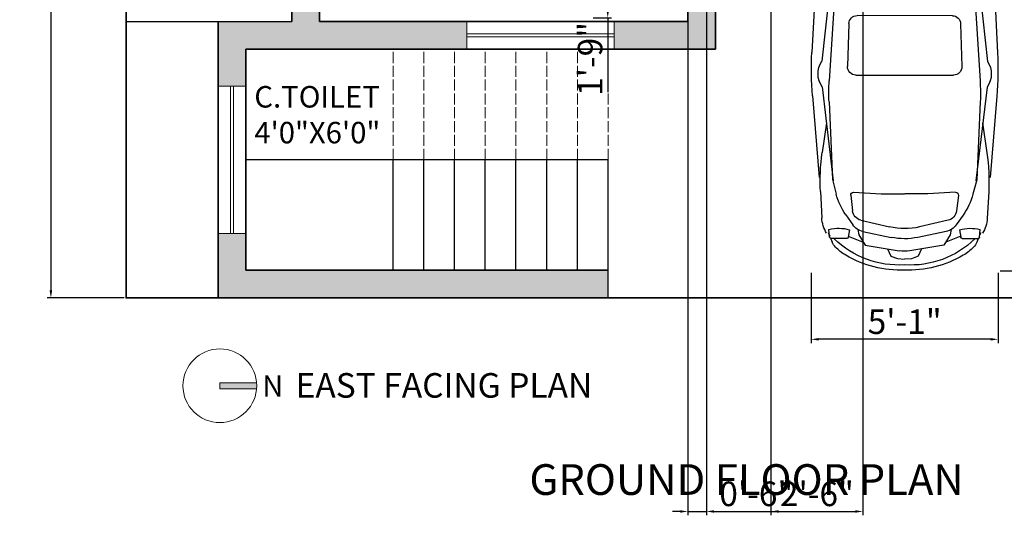
# Model space of a CAD drawing. Units: inches. Extents: x 4732 to 5926, y 2665 to 3255.
# Tile 1 of 8: x 4784 to 5104, y 2665 to 2827. Entities that reach past the tile are written whole.
import ezdxf

# ---------------------------------------------------------------- set-up
doc = ezdxf.new("R2010")
doc.units = ezdxf.units.IN
doc.linetypes.add('ACAD_ISO02W100', pattern=[15, 12, -3])
for name, color, linetype, lineweight in [('A-ANNO-DIMS', 2, 'Continuous', 18), ('A-ANNO-SYMB', 7, 'Continuous', 18), ('A-ANNO-TITL', 7, 'Continuous', 25), ('A-AREA-IDEN', 7, 'Continuous', 18), ('A-FLOR', 7, 'Continuous', 25), ('A-FLOR-STRS', 7, 'Continuous', 25), ('A-FLOR-STRS-HIDN', 8, 'ACAD_ISO02W100', 18), ('A-GLAZ', 4, 'Continuous', 18), ('A-SITE-VEHS', 8, 'Continuous', 13), ('A-WALL', 7, 'Continuous', 35), ('A-WALL-PATT', 8, 'Continuous', 13), ('C-PROP', 7, 'Continuous', 35)]:
    doc.layers.add(name, color=color, linetype=linetype, lineweight=lineweight)
doc.layers.add('L9012X$0', color=2, linetype='Continuous')
doc.styles.get("Standard").update_dxf_attribs({"font": 'arial.ttf'})
doc.dimstyles.new('ISO-25', dxfattribs={"dimtxt": 8, "dimasz": 2.5, "dimexe": 1.25, "dimexo": 0.625, "dimtad": 1, "dimdec": 1, "dimlunit": 3, "dimtxsty": 'Standard', "dimcen": 2.5, "dimadec": 0, "dimazin": 0, "dimtfac": 1, "dimtdec": 1, "dimtmove": 0, "dimatfit": 3, "dimfxl": 1, "dimarcsym": 0})

# ---------------------------------------------------------------- blocks, each defined once
blk = doc.blocks.new('A1099DC')
at = {"color": 0, "linetype": 'ByBlock'}
for p, q in [((1279.298465, 804.448389), (2201.430588, 851.890505)), ((2602.736326, 846.078152), (3356.693814, 785.353187)), ((272.228253, 749.073842), (265.114727, 718.465169)), ((1475.52921, 670.226262), (2282.402739, 758.004075)), ((2519.280414, 756.817792), (3387.476361, 653.818028)), ((2851.341839, 715.213377), (3126.60716, 755.701993)), ((3488.458929, 772.663345), (3732.658862, 759.86454)), ((139.051458, 595.027331), (190.951238, 683.213377)), ((179.200345, 564.515703), (190.951238, 709.631982)), ((398.733388, 644.315148), (411.280494, 678.748261)), ((411.280494, 678.748261), (588.616917, 641.417897)), ((1482.852352, 674.283145), (1175.286956, 622.180789)), ((1494.603245, 682.841284), (1678.210958, 641.166865)), ((1678.210958, 641.166865), (2462.684993, 690.847736)), ((2656.476214, 692.831247), (3376.704709, 662.004075)), ((3376.704709, 662.004075), (3510.708679, 626.736433)), ((3909.27561, 688.812956), (3837.725727, 693.401722)), ((3867.794139, 700.329656), (3900.059395, 686.767505)), ((3921.162781, 527.618662), (3921.162781, 676.138994)), ((3925.383812, 676.122818), (3955.306409, 663.545364)), ((92.537504, 388.14361), (139.051458, 595.027331)), ((236.043912, 551.980927), (179.200345, 564.515703)), ((405.405047, 577.538958), (396.874865, 615.894428)), ((589.014326, 626.599587), (405.405047, 577.538958)), ((1300.814287, 466.658131), (1445.712032, 613.104998)), ((1465.665584, 620.56924), (1602.893878, 610.287296)), ((1626.354615, 583.507504), (1602.652901, 169.222264)), ((229.117398, 477.634662), (225.714299, 427.957563)), ((1933.148906, 509.557888), (2330.980062, 522.200075)), ((3493.960271, 465.734554), (3507.923021, 209.166865)), ((3522.252709, 492.345257), (3666.066199, 475.644444)), ((3704.596898, 536.993674), (3795.675135, 473.385795)), ((3841.786866, 503.451367), (3910.58243, 515.096797)), ((3901.001848, 514.780764), (3957.150905, 375.772812)), ((57.774444, 216.608726), (92.537504, 388.14361)), ((1235.045743, 136.116317), (1257.419842, 373.755108)), ((1860.238743, -448.635916), (1859.369151, 433.397797)), ((2409.60024, 445.938054), (2410.49349, -460.09121)), ((3753.293176, 397.789551), (3815.226005, 132.124765)), ((3839.396146, 426.841284), (3888.358202, 417.538958)), ((3857.610793, 379.525702), (3912.067615, 118.157673)), ((3888.358202, 417.538958), (3983.199613, 359.957848)), ((3983.199613, 359.957848), (4035.448301, 43.94997)), ((49.168662, 58.00681), (57.774444, 216.608726)), ((3507.923021, 209.166865), (3507.64153, -4.333678)), ((4019.086894, 150.376168), (4084.69605, 122.469191)), ((4084.69605, 122.469191), (4109.177079, 60.329656)), ((4109.177079, 60.329656), (4113.094043, -5.158716)), ((49.301278, -76.507426), (58.219773, -235.092064)), ((3508.347273, -221.154823), (3507.644805, -7.65525)), ((3983.920268, -371.008369), (4035.545755, -54.898082)), ((4084.948231, -133.320044), (4109.306686, -71.132359)), ((4109.306686, -71.132359), (4113.094514, -5.636391)), ((1235.330373, -152.586046), (1258.173002, -390.180259)), ((3754.088875, -409.293325), (3815.497749, -143.506937)), ((3858.370276, -390.823819), (3912.311631, -129.348921)), ((4019.394229, -161.356334), (4084.948231, -133.320044)), ((58.219773, -235.092064), (93.320996, -406.558069)), ((1627.520644, -599.204785), (1603.002095, -184.967086)), ((3494.890446, -477.749545), (3508.347273, -221.154823)), ((93.320996, -406.558069), (140.24279, -613.349673)), ((230.077082, -495.779641), (226.576036, -446.109349)), ((3840.248961, -438.175225), (3889.19258, -428.776374)), ((3889.19258, -428.776374), (3983.920268, -371.008369)), ((3902.027941, -525.993061), (3957.902795, -386.874665)), ((1301.750547, -482.997536), (1446.936772, -629.158411)), ((1934.168526, -524.650381), (2332.023837, -536.508105)), ((3523.2353, -504.304409), (3667.01558, -487.320059)), ((3705.667171, -548.593196), (3796.61981, -484.805853)), ((3842.790735, -514.780444), (3911.609128, -526.290202)), ((3922.214148, -538.79118), (3922.506998, -687.311224)), ((140.24279, -613.349673), (192.316354, -701.433212)), ((237.150178, -570.112104), (180.331436, -582.758939)), ((180.331436, -582.758939), (192.368445, -727.851766)), ((406.561378, -595.336142), (398.106841, -633.708356)), ((590.267037, -644.034637), (406.561378, -595.336142)), ((1466.905004, -636.583294), (1604.112757, -626.030785)), ((400.0214, -662.125356), (412.636377, -696.533662)), ((412.636377, -696.533662), (589.898847, -658.853701)), ((1484.19765, -690.263206), (1176.530118, -638.767405)), ((1476.866524, -686.22077), (2283.911563, -772.40743)), ((1495.965396, -698.798158), (1679.490579, -656.761786)), ((1679.490579, -656.761786), (2464.061049, -704.895745)), ((2520.786439, -770.754078), (3388.777604, -666.042617)), ((2657.855804, -706.497136), (3378.022114, -674.249887)), ((2852.765183, -728.494989), (3128.109803, -768.440762)), ((3378.022114, -674.249887), (3511.956283, -638.718087)), ((3910.644841, -700.0086), (3839.104145, -704.738438)), ((3869.186159, -711.60707), (3901.424611, -697.981326)), ((3926.727989, -687.286725), (3956.625729, -674.650294)), ((273.723073, -767.133288), (266.549207, -736.538701)), ((2604.418191, -859.849707), (3358.254477, -797.638217)), ((3489.994314, -784.688586), (3734.168535, -771.408296)), ((1280.900818, -820.829563), (2203.124693, -866.453338))]:
    blk.add_line(p, q, dxfattribs=at)
for points in [[(-0.000783, 0.794772), (5.385043, 172.701749), (63.649891, 493.818028), (92.537504, 603.957563), (144.437284, 705.166865), (428.417214, 824.236633), (585.095796, 846.190121), (961.406447, 846.190121), (1274.27399, 797.818028), (1482.852352, 709.631982)], [(83.345007, -3.206171), (111.32237, 268.957533), (164.563706, 379.583828), (279.999271, 453.709838), (456.549665, 511.628518), (901.254996, 574.918954), (1175.286956, 622.180789), (1137.52997, 385.548359), (1118.345181, 137.317882), (1109.829198, -8.358455)], [(168.178729, 359.003083), (1030.214866, 528.397865), (1077.798844, 510.531569), (1086.170082, 475.285426), (992.832238, 91.960378), (924.218938, 35.478085), (108.447994, 6.034416)], [(0.019119, -19.392451), (5.743899, -191.288474), (64.641806, -512.289243), (93.746535, -622.371603), (145.845778, -723.478374), (430.059935, -841.987962), (586.7815, -863.632471), (963.091723, -863.198028), (1275.863278, -814.209121), (1484.26735, -725.611974)], [(83.356858, -15.227176), (111.870816, -287.335185), (165.330179, -397.856284), (280.911681, -471.754535), (457.575935, -529.324983), (902.4055, -592.045995), (1176.530118, -638.767405), (1138.306616, -402.209884), (1118.632407, -154.017717), (1109.829198, -8.358455)], [(168.904615, -377.268451), (1031.273389, -545.270714), (1078.822046, -527.310627), (1087.123771, -492.048047), (993.030273, -108.907787), (924.305735, -52.560894), (108.478017, -24.418246)]]:
    blk.add_lwpolyline(points, dxfattribs=at)
for centre, radius, start, end in [((2358.037832, -2192.08357), 3048, 85.395244, 92.945173), ((2399.99649, 588.663508), 206.166238, 54.649181, 124.776949), ((3392.740754, -1053.630025), 1828.8, 86.999806, 98.367602), ((3718.678317, 475.802507), 284.405862, 57.329946, 87.182375), ((1749.553982, 373.478072), 1524, 166.916578, 176.08111), ((446.46332, 626.922805), 50.8, 159.97873, 192.538409), ((587.047263, 633.961317), 7.62, 284.960009, 78.112462), ((2578.271641, -1134.295865), 1828.8, 87.549126, 93.623712), ((4191.049821, 605.937201), 363.988953, 166.096081, 196.353514), ((3908.462781, 676.138994), 12.7, 0, 86.330429), ((3320.85101, 50.338397), 847.430844, 356.245089, 44.519453), ((3896.252417, 523.051998), 152.4, 46.38363, 67.20138), ((1463.767788, 595.240237), 25.4, 85.715073, 135.304647), ((1600.996082, 584.958293), 25.4, 356.725615, 85.715073), ((3355.555414, 37.211519), 609.6, 55.070043, 75.255062), ((3700.933354, 318.064082), 435.542335, 30.457681, 46.38363), ((1409.148822, 359.469565), 152.4, 135.304647, 174.62136), ((1935.569151, 433.396333), 76.2, 91.82012, 179.9989), ((2333.400307, 446.03852), 76.2, 359.924458, 91.82012), ((3519.322741, 467.114813), 25.4, 83.37601, 183.115039), ((3654.346327, 374.722669), 101.6, 13.122645, 83.37601), ((3708.414764, 348.440256), 152.4, 11.769371, 55.070043), ((3908.462781, 527.618662), 12.7, 279.607718, 0), ((3204.184594, 25.950693), 1011.814461, 358.069446, 30.457681), ((2752.335538, -6.739118), 1524, 174.62136, 185.491615), ((4645.676894, -4.872483), 3048, 176.725615, 183.38736), ((3221.54491, -6.276527), 609.6, 346.99033, 13.122645), ((3315.283499, -6.18411), 609.6, 348.343604, 11.769371), ((1266.577845, -8.050136), 1219.2, 176.894161, 183.218814), ((3734.73098, -5.770579), 304.8, 350.724636, 9.388339), ((3320.962449, -62.69553), 847.430844, 315.593523, 3.867886), ((3204.248172, -38.537915), 1011.814461, 329.655294, 2.043529), ((1409.873518, -375.595566), 152.4, 185.491615, 224.808328), ((1936.438592, -448.484202), 76.2, 180.114076, 268.292856), ((3655.096735, -386.42159), 101.6, 276.736965, 346.99033), ((3709.113243, -360.032616), 152.4, 305.042932, 348.343604), ((1750.305335, -388.625277), 1524, 184.031865, 193.196397), ((2334.293902, -460.341926), 76.2, 268.292856, 0.188517), ((3520.255588, -479.079792), 25.4, 176.997936, 276.736965), ((4192.255091, -616.577407), 363.988953, 163.759461, 194.016894), ((3909.514173, -538.816222), 12.7, 0.112975, 80.505257), ((447.716945, -644.638934), 50.8, 167.574566, 200.134245), ((1464.957267, -611.258083), 25.4, 224.808328, 274.397903), ((1602.165021, -600.705574), 25.4, 274.397903, 3.38736), ((3355.640902, -49.500248), 609.6, 284.857913, 305.042932), ((3701.571953, -329.671253), 435.542335, 313.729345, 329.655294), ((588.314493, -651.400231), 7.62, 282.000513, 75.152966), ((2576.048678, 1120.472221), 1828.8, 266.489263, 272.563849), ((3719.627907, -487.374382), 284.405862, 272.930601, 302.78303), ((3909.807023, -687.336265), 12.7, 273.782546, 0.112975), ((3897.294828, -534.273643), 152.4, 292.911596, 313.729345), ((2401.171182, -602.835323), 206.166238, 235.336026, 305.463794), ((3390.675263, 1041.412497), 1828.8, 261.745373, 273.113169), ((2353.729565, 2177.823616), 3048, 267.167802, 274.717731)]:
    blk.add_arc(centre, radius, start, end, dxfattribs=at)
blk = doc.blocks.new('VI')
at = {"layer": 'L9012X$0'}
blk.add_blockref('A1099DC', (0, 0), dxfattribs=at)
blk = doc.blocks.new('*D28')
at = {"layer": 'A-ANNO-DIMS', "color": 0, "lineweight": -2, "transparency": 16777216}
for p, q in [((4817.76, 3215.93), (4792.67, 3215.93)), ((4793.92, 3213.43), (4793.92, 2738.43)), ((4817.76, 2735.93), (4792.67, 2735.93))]:
    blk.add_line(p, q, dxfattribs=at)
at = {"layer": 'A-ANNO-DIMS', "color": 0, "transparency": 16777216}
for points in [[(4793.5, 3213.43), (4794.33, 3213.43), (4793.92, 3215.93)], [(4793.5, 2738.43), (4794.33, 2738.43), (4793.92, 2735.93)]]:
    blk.add_solid(points, dxfattribs=at)
at = {"layer": 'Defpoints', "color": 0, "transparency": 16777216}
for p in [(4818.38, 3215.93), (4793.92, 2735.93), (4818.38, 2735.93)]:
    blk.add_point(p, dxfattribs=at)
at = {"layer": 'A-ANNO-DIMS', "color": 0, "transparency": 16777216, "insert": (4789.21, 2975.93), "char_height": 8, "attachment_point": 5, "rotation": 90}
blk.add_mtext("40'", dxfattribs=at)
blk = doc.blocks.new('GLAZ-UNIT-48IN')
for p, q in [((0, 1), (48, 1)), ((0, 0), (48, 0))]:
    blk.add_line(p, q)
blk = doc.blocks.new('NORTH-INDICATOR')
at = {"transparency": 33554687}
h = blk.add_hatch(color=256, dxfattribs=at)
h.dxf.hatch_style = 1
h.paths.add_polyline_path([(0, 1), (0, -1), (11.96, -1, 0.020861), (12, 0, 0.020861), (11.96, 1)])
for p, q in [((0, -1), (0, 1)), ((0, 1), (11.96, 1)), ((12, -1), (0, -1))]:
    blk.add_line(p, q)
blk.add_circle((0, 0), 12)
blk.add_text('N', height=6.9).set_placement((13.83, -3.53))
blk = doc.blocks.new('*D85')
at = {"layer": 'A-ANNO-DIMS', "color": 0, "lineweight": -2, "transparency": 16777216}
for p, q in [((4970.49, 2848.15), (4976.52, 2848.15)), ((4975.27, 2845.65), (4975.27, 2829.65)), ((4970.49, 2827.15), (4976.52, 2827.15)), ((4975.27, 2827.15), (4975.27, 2802.89))]:
    blk.add_line(p, q, dxfattribs=at)
at = {"layer": 'A-ANNO-DIMS', "color": 0, "transparency": 16777216}
for points in [[(4974.85, 2845.65), (4975.69, 2845.65), (4975.27, 2848.15)], [(4974.85, 2829.65), (4975.69, 2829.65), (4975.27, 2827.15)]]:
    blk.add_solid(points, dxfattribs=at)
at = {"layer": 'Defpoints', "color": 0, "transparency": 16777216}
for p in [(4969.87, 2848.15), (4969.87, 2827.15), (4975.27, 2827.15)]:
    blk.add_point(p, dxfattribs=at)
at = {"layer": 'A-ANNO-DIMS', "color": 0, "transparency": 16777216, "insert": (4970.56, 2813.77), "char_height": 8, "attachment_point": 5, "rotation": 90}
blk.add_mtext('1\'-9"', dxfattribs=at)
blk = doc.blocks.new('*D96')
at = {"layer": 'A-ANNO-DIMS', "color": 0, "lineweight": -2, "transparency": 16777216}
for p, q in [((5103.06, 2893.31), (5125.97, 2893.31)), ((5124.72, 2890.81), (5124.72, 2747.23)), ((5103.06, 2744.73), (5125.97, 2744.73))]:
    blk.add_line(p, q, dxfattribs=at)
at = {"layer": 'A-ANNO-DIMS', "color": 0, "transparency": 16777216}
for points in [[(5124.3, 2890.81), (5125.14, 2890.81), (5124.72, 2893.31)], [(5124.3, 2747.23), (5125.14, 2747.23), (5124.72, 2744.73)]]:
    blk.add_solid(points, dxfattribs=at)
at = {"layer": 'Defpoints', "color": 0, "transparency": 16777216}
for p in [(5102.43, 2893.31), (5102.43, 2744.73), (5124.72, 2744.73)]:
    blk.add_point(p, dxfattribs=at)
at = {"layer": 'A-ANNO-DIMS', "color": 0, "transparency": 16777216, "insert": (5119.96, 2819.02), "char_height": 8, "attachment_point": 5, "rotation": 90}
blk.add_mtext('CAR 12\'-4 1/2"', dxfattribs=at)
blk = doc.blocks.new('*D97')
at = {"layer": 'A-ANNO-DIMS', "color": 0, "lineweight": -2, "transparency": 16777216}
for p, q in [((5041.49, 2744.1), (5041.49, 2721.19)), ((5102.43, 2744.1), (5102.43, 2721.19)), ((5099.93, 2722.44), (5043.99, 2722.44))]:
    blk.add_line(p, q, dxfattribs=at)
at = {"layer": 'A-ANNO-DIMS', "color": 0, "transparency": 16777216}
for points in [[(5043.99, 2722.86), (5043.99, 2722.03), (5041.49, 2722.44)], [(5099.93, 2722.86), (5099.93, 2722.03), (5102.43, 2722.44)]]:
    blk.add_solid(points, dxfattribs=at)
at = {"layer": 'Defpoints', "color": 0, "transparency": 16777216}
for p in [(5041.49, 2744.73), (5102.43, 2744.73), (5041.49, 2722.44)]:
    blk.add_point(p, dxfattribs=at)
at = {"layer": 'A-ANNO-DIMS', "color": 0, "transparency": 16777216, "insert": (5071.96, 2727.15), "char_height": 8, "attachment_point": 5}
blk.add_mtext('5\'-1"', dxfattribs=at)
blk = doc.blocks.new('*D107')
at = {"layer": 'A-ANNO-DIMS', "color": 0, "lineweight": -2, "transparency": 16777216}
for p, q in [((5028.38, 3098.31), (5028.38, 2665.12)), ((5058.38, 3098.31), (5058.38, 2665.12)), ((5030.88, 2666.37), (5055.88, 2666.37))]:
    blk.add_line(p, q, dxfattribs=at)
at = {"layer": 'A-ANNO-DIMS', "color": 0, "transparency": 16777216}
for points in [[(5030.88, 2666.79), (5030.88, 2665.96), (5028.38, 2666.37)], [(5055.88, 2666.79), (5055.88, 2665.96), (5058.38, 2666.37)]]:
    blk.add_solid(points, dxfattribs=at)
at = {"layer": 'Defpoints', "color": 0, "transparency": 16777216}
for p in [(5028.38, 3098.93), (5058.38, 3098.93), (5058.38, 2666.37)]:
    blk.add_point(p, dxfattribs=at)
at = {"layer": 'A-ANNO-DIMS', "color": 0, "transparency": 16777216, "insert": (5043.38, 2671.08), "char_height": 8, "attachment_point": 5}
blk.add_mtext('2\'-6"', dxfattribs=at)
blk = doc.blocks.new('*D114')
at = {"layer": 'A-ANNO-DIMS', "color": 0, "lineweight": -2, "transparency": 16777216}
for p, q in [((5007.38, 3104.31), (5007.38, 2665.12)), ((5001.38, 3098.31), (5001.38, 2665.12)), ((4998.88, 2666.37), (4996.38, 2666.37)), ((5001.38, 2666.37), (5007.38, 2666.37)), ((5009.88, 2666.37), (5034.9, 2666.37))]:
    blk.add_line(p, q, dxfattribs=at)
at = {"layer": 'A-ANNO-DIMS', "color": 0, "transparency": 16777216}
for points in [[(4998.88, 2666.79), (4998.88, 2665.96), (5001.38, 2666.37)], [(5009.88, 2666.79), (5009.88, 2665.96), (5007.38, 2666.37)]]:
    blk.add_solid(points, dxfattribs=at)
at = {"layer": 'Defpoints', "color": 0, "transparency": 16777216}
for p in [(5007.38, 3104.93), (5001.38, 3098.93), (5007.38, 2666.37)]:
    blk.add_point(p, dxfattribs=at)
at = {"layer": 'A-ANNO-DIMS', "color": 0, "transparency": 16777216, "insert": (5023.64, 2671.08), "char_height": 8, "attachment_point": 5}
blk.add_mtext('0\'-6"', dxfattribs=at)

msp = doc.modelspace()

# ---------------------------------------------------------------- hatches: boundary and pattern name
at = {"layer": 'A-WALL-PATT'}
h = msp.add_hatch(color=256, dxfattribs=at)
h.dxf.hatch_style = 1
h.paths.add_polyline_path([(4905.38, 3185.93), (4848.38, 3185.93), (4848.38, 3146.93), (4857.38, 3146.93), (4857.38, 3176.93), (4905.38, 3176.93)])
h.paths.add_polyline_path([(5022.38, 3185.93), (4953.38, 3185.93), (4953.38, 3176.93), (4966.1, 3176.93), (5001.38, 3176.93), (5001.38, 3098.93), (5028.38, 3098.93), (5028.38, 3104.93), (5007.38, 3104.93), (5007.38, 3176.93), (5022.38, 3176.93)])
h.paths.add_polyline_path([(5115.38, 3185.93), (5046.38, 3185.93), (5046.38, 3176.93), (5061.38, 3176.93), (5061.38, 3104.93), (5058.38, 3104.93), (5058.38, 3098.93), (5067.38, 3098.93), (5067.38, 3176.93), (5115.38, 3176.93)])
h.paths.add_polyline_path([(5220.38, 3185.93), (5163.38, 3185.93), (5163.38, 3176.93), (5168.97, 3176.93), (5211.38, 3176.93), (5211.38, 3146.93), (5220.38, 3146.93)])
h.paths.add_polyline_path([(4857.38, 3086.93), (4848.38, 3086.93), (4848.38, 3026.93), (4857.38, 3026.93), (4857.38, 3050.93), (5001.38, 3050.93), (5001.38, 3008.93), (5007.38, 3008.93), (5007.38, 3050.93), (5022.38, 3050.93), (5022.38, 3056.93), (4857.38, 3056.93)])
h.paths.add_polyline_path([(4857.38, 2978.93), (4848.38, 2978.93), (4848.38, 2945.93), (4872.38, 2945.93), (4872.38, 2933.93), (4875.38, 2933.93), (4881.38, 2933.93), (4881.38, 2954.93), (4857.38, 2954.93)])
h.paths.add_polyline_path([(4881.38, 2903.93), (4875.38, 2903.93), (4872.38, 2903.93), (4872.38, 2897.93), (4881.38, 2897.93)])
h.paths.add_polyline_path([(4881.38, 2849.93), (4872.38, 2849.93), (4872.38, 2828.75), (4872.38, 2825.93), (4848.38, 2825.93), (4848.38, 2804.93), (4857.38, 2804.93), (4857.38, 2816.93), (4929.38, 2816.93), (4929.38, 2825.93), (4881.38, 2825.93)])
h.paths.add_polyline_path([(4975.38, 2744.93), (4857.38, 2744.93), (4857.38, 2756.93), (4848.38, 2756.93), (4848.38, 2735.93), (4975.38, 2735.93)])
h.paths.add_polyline_path([(5160.38, 2915.93), (5160.38, 2918.93), (5007.38, 2918.93), (5007.38, 2960.93), (5001.38, 2960.93), (5001.38, 2825.93), (4977.38, 2825.93), (4977.38, 2816.93), (5010.38, 2816.93), (5010.38, 2909.93), (5160.38, 2909.93)])
h.paths.add_polyline_path([(5220.38, 2948.93), (5211.38, 2948.93), (5211.38, 2918.93), (5208.38, 2918.93), (5208.38, 2909.93), (5220.38, 2909.93)])
h.paths.add_polyline_path([(5220.38, 3086.93), (5211.38, 3086.93), (5211.38, 3056.93), (5106.38, 3056.93), (5106.38, 3050.93), (5211.38, 3050.93), (5211.38, 3020.93), (5220.38, 3020.93)])
h.paths.add_polyline_path([(5067.38, 3098.93), (5061.38, 3098.93), (5061.38, 3056.93), (5058.38, 3056.93), (5058.38, 3050.93), (5061.38, 3050.93), (5070.38, 3050.93), (5070.38, 3056.93), (5067.38, 3056.93)])
h.paths.add_polyline_path([(4883.76, 2941.13), (4938.24, 2941.13), (4938.24, 2949.38), (4883.76, 2949.38)], flags=9)
h.paths.add_polyline_path([(4840.48, 3026.79), (4840.48, 3093.88), (4825.54, 3093.88), (4825.54, 3026.79)], flags=9)
h.paths.add_polyline_path([(5245.66, 2994.98), (5245.66, 3062.07), (5230.72, 3062.07), (5230.72, 2994.98)], flags=9)
h.paths.add_polyline_path([(4994.89, 3193.24), (5061.99, 3193.24), (5061.99, 3208.18), (4994.89, 3208.18)], flags=9)
h.paths.add_polyline_path([(5081.53, 3115.35), (5081.53, 3161.13), (5073.28, 3161.13), (5073.28, 3115.35)], flags=25)
h.paths.add_polyline_path([(4997.53, 3115.35), (4997.53, 3161.13), (4989.28, 3161.13), (4989.28, 3115.35)], flags=25)
h.paths.add_polyline_path([(5175.31, 2866.04), (5202.42, 2866.04), (5202.42, 2876.71), (5175.31, 2876.71)], flags=9)
h.paths.add_polyline_path([(4820.13, 2876.28), (4869.1, 2876.28), (4869.1, 2902.89), (4820.13, 2902.89)], flags=9)
h.paths.add_polyline_path([(5104.69, 2868.81), (5158.82, 2868.81), (5158.82, 2895.42), (5104.69, 2895.42)], flags=25)
h.paths.add_polyline_path([(5084.11, 2966.75), (5138.25, 2966.75), (5138.25, 2993.36), (5084.11, 2993.36)], flags=9)
h.paths.add_polyline_path([(4897.84, 3000.24), (4946.81, 3000.24), (4946.81, 3026.85), (4897.84, 3026.85)], flags=9)
h.paths.add_polyline_path([(5009.53, 3133.48), (5059.32, 3133.48), (5059.32, 3160.09), (5009.53, 3160.09)], flags=9)
h.paths.add_polyline_path([(5124.24, 3088.37), (5180.47, 3088.37), (5180.47, 3114.99), (5124.24, 3114.99)], flags=9)
h.paths.add_polyline_path([(4897.52, 3088.37), (4965.52, 3088.37), (4965.52, 3114.99), (4897.52, 3114.99)], flags=9)
h.paths.add_polyline_path([(4924.5, 2879.19), (4978.63, 2879.19), (4978.63, 2905.8), (4924.5, 2905.8)], flags=9)

# ---------------------------------------------------------------- linework, layer by layer
at = {"layer": 'A-FLOR'}
msp.add_line((4818.38, 2825.93), (4872.38, 2825.93), dxfattribs=at)
at = {"layer": 'A-FLOR-STRS'}
for p, q in [((4975.38, 2780.93), (4857.38, 2780.93)), ((4905.38, 2744.93), (4905.38, 2780.93)), ((4915.38, 2744.93), (4915.38, 2780.93)), ((4925.38, 2744.93), (4925.38, 2780.93)), ((4935.38, 2744.93), (4935.38, 2780.93)), ((4945.38, 2744.93), (4945.38, 2780.93)), ((4955.38, 2744.93), (4955.38, 2780.93)), ((4965.38, 2744.93), (4965.38, 2780.93)), ((4975.38, 2735.93), (4975.38, 2780.93))]:
    msp.add_line(p, q, dxfattribs=at)
at = {"layer": 'A-FLOR-STRS-HIDN', "ltscale": 0.3}
for p, q in [((4905.38, 2780.93), (4905.38, 2816.93)), ((4915.38, 2780.93), (4915.38, 2816.93)), ((4925.38, 2780.93), (4925.38, 2816.93)), ((4935.38, 2780.93), (4935.38, 2816.93)), ((4945.38, 2780.93), (4945.38, 2816.93)), ((4955.38, 2780.93), (4955.38, 2816.93)), ((4965.38, 2780.93), (4965.38, 2816.93)), ((4975.38, 2780.93), (4975.38, 2816.93))]:
    msp.add_line(p, q, dxfattribs=at)
at = {"layer": 'A-GLAZ'}
for p, q in [((4929.38, 2816.93), (4929.38, 2825.93)), ((4977.38, 2816.93), (4977.38, 2825.93)), ((4857.38, 2804.93), (4848.38, 2804.93)), ((4857.38, 2756.93), (4848.38, 2756.93))]:
    msp.add_line(p, q, dxfattribs=at)
at = {"layer": 'A-WALL'}
for p, q in [((5001.38, 2825.93), (5001.38, 2960.93)), ((5010.38, 2816.93), (5010.38, 2909.93)), ((4872.38, 2825.93), (4872.38, 2903.93)), ((4881.38, 2825.93), (4881.38, 2903.93)), ((4848.38, 2735.93), (4848.38, 2825.93)), ((4881.38, 2825.93), (5001.38, 2825.93)), ((4857.38, 2744.93), (4857.38, 2816.93)), ((4857.38, 2816.93), (5010.38, 2816.93)), ((4975.38, 2744.93), (4857.38, 2744.93))]:
    msp.add_line(p, q, dxfattribs=at)
at = {"layer": 'C-PROP'}
msp.add_lwpolyline([(4818.38, 3215.93), (5250.38, 3215.93), (5250.38, 2735.93), (4818.38, 2735.93)], close=True, dxfattribs=at)

# ---------------------------------------------------------------- block references
at = {"layer": 'A-ANNO-SYMB'}
msp.add_blockref('NORTH-INDICATOR', (4848.93, 2707.32), dxfattribs=at)
at = {"layer": 'A-GLAZ'}
for p, rotation in [((4977.38, 2821.93), 180), ((4852.38, 2804.93), 269.9999999999978)]:
    msp.add_blockref('GLAZ-UNIT-48IN', p, dxfattribs=dict(at, rotation=rotation))
at = {"layer": 'A-SITE-VEHS', "xscale": -0.0351896714874634, "yscale": 0.0351896714874634, "zscale": 0.0351896714874634, "rotation": 90}
msp.add_blockref('VI', (5071.71, 2893.31), dxfattribs=at)

# ---------------------------------------------------------------- texts
at = {"layer": 'A-ANNO-TITL', "attachment_point": 1}
for s, insert, char_height in [('{\\fTimes New Roman|b0|i0|c0|p18;EAST FACING PLAN}', (4873.62, 2711.44), 8), ('{\\fTimes New Roman|b0|i0|c0|p18;GROUND FLOOR PLAN}', (4949.75, 2681.77), 10)]:
    msp.add_mtext_dynamic_manual_height_columns(s, width=196.2607, gutter_width=12.5, heights=[0], dxfattribs=dict(at, insert=insert, char_height=char_height))
at = {"layer": 'A-AREA-IDEN', "insert": (4860.16, 2804.93), "char_height": 7, "attachment_point": 1}
msp.add_mtext_dynamic_manual_height_columns('{\\fTimes New Roman|b0|i0|c0|p18;C.TOILET\\P4\'0"X6\'0"}', width=61.0557, gutter_width=12.5, heights=[0], dxfattribs=at)

# ---------------------------------------------------------------- dimensions: what is measured, and where the dimension line sits
at = {"layer": 'A-ANNO-DIMS'}
for base, p1, p2, angle, override, picture, middle in [((4793.92, 2735.93), (4818.38, 3215.93), (4818.38, 2735.93), 90, {"dimclrd": 0, "dimclre": 0, "dimclrt": 0}, '*D28', (4789.21, 2975.93)), ((4975.27, 2827.15), (4969.87, 2848.15), (4969.87, 2827.15), 270, {"dimdec": 1, "dimlfac": 1, "dimrnd": 0, "dimzin": 1, "dimdsep": 46, "dimlunit": 4, "dimfrac": 2}, '*D85', (4970.56, 2813.77)), ((5041.49, 2722.44), (5102.43, 2744.73), (5041.49, 2744.73), 180, {"dimdec": 1, "dimlfac": 1, "dimrnd": 0, "dimzin": 1, "dimdsep": 46, "dimlunit": 4, "dimfrac": 2}, '*D97', (5071.96, 2727.15))]:
    dim = msp.add_linear_dim(base=base, p1=p1, p2=p2, angle=angle, dimstyle='ISO-25', override=override, dxfattribs=at)
    dim.commit()
    dim.dimension.update_dxf_attribs({"geometry": picture, "text_midpoint": middle})
for base, p1, p2, picture, middle in [((5007.38, 2666.37), (5001.38, 3098.93), (5007.38, 3104.93), '*D114', (5023.64, 2671.08)), ((5058.38, 2666.37), (5028.38, 3098.93), (5058.38, 3098.93), '*D107', (5043.38, 2671.08))]:
    dim = msp.add_linear_dim(base=base, p1=p1, p2=p2, dimstyle='ISO-25', override={"dimdec": 1, "dimlfac": 1, "dimrnd": 0, "dimzin": 1, "dimdsep": 46, "dimlunit": 4, "dimfrac": 2}, dxfattribs=at)
    dim.commit()
    dim.dimension.update_dxf_attribs({"geometry": picture, "text_midpoint": middle})
dim = msp.add_linear_dim(base=(5124.72, 2744.73), p1=(5102.43, 2893.31), p2=(5102.43, 2744.73), angle=270, text='CAR <>', dimstyle='ISO-25', override={"dimdec": 1, "dimlfac": 1, "dimrnd": 0, "dimzin": 1, "dimdsep": 46, "dimlunit": 4, "dimfrac": 2}, dxfattribs=at)
dim.commit()
dim.dimension.update_dxf_attribs({"geometry": '*D96', "text_midpoint": (5119.96, 2819.02)})

doc.saveas('drawing.dxf')
